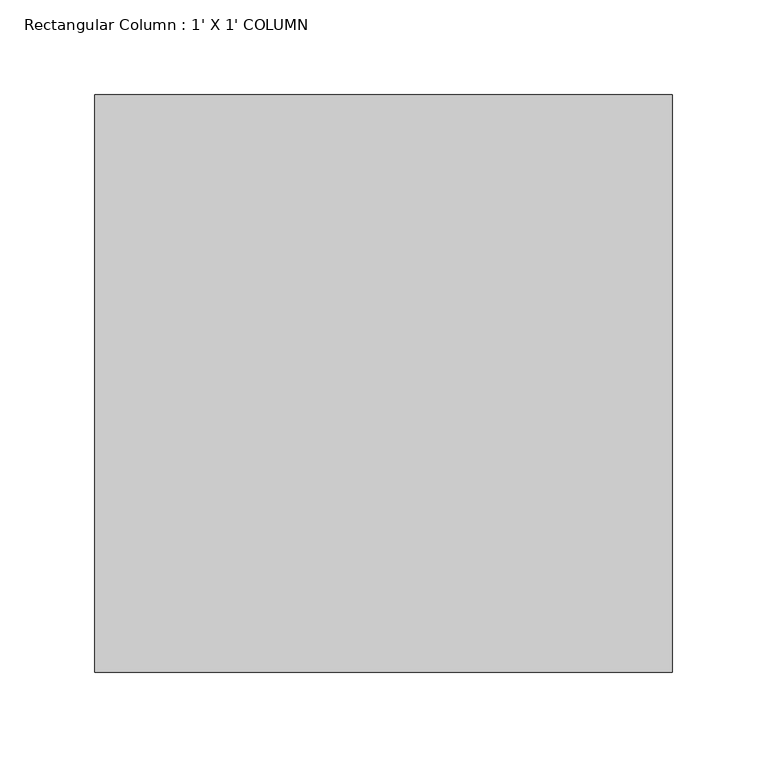
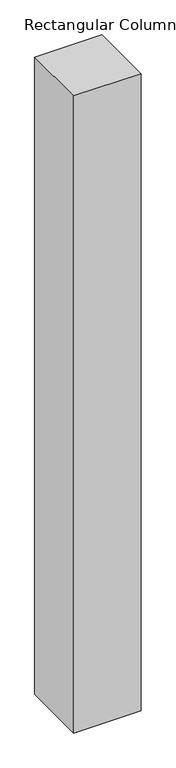
"""IFC4 building model written with IfcOpenShell, lengths in millimetres: column geometry, Rectangular Column : 1' X 1' COLUMN."""

from ifc_helpers import new_model, si_unit, origin, origin_with_axes, place, context, project, spatial, polyline, outline, extrude, source, transform, mapped, element, save


def rectangular_column_1_x_1_column_d780e21f(model_context):
    return source(origin(), model_context, "Body", "SweptSolid", [
        extrude(outline(polyline([(152.4, 152.4), (152.4, -152.4), (-152.4, -152.4), (-152.4, 152.4), (152.4, 152.4)])), origin_with_axes(), (0.0, 0.0, 1.0), 3048.0),
    ])


if __name__ == "__main__":
    model = new_model("IFC4")
    model_context = context("Model", 3, world=origin())
    ifc_project = project(units=[si_unit("LENGTHUNIT", "METRE", prefix="MILLI")], contexts=[model_context])
    site = spatial("IfcSite", under=ifc_project)
    building = spatial("IfcBuilding", under=site)
    placement = place(None, origin())
    rectangular_column_1_x_1_column_shape = rectangular_column_1_x_1_column_d780e21f(model_context)
    element("IfcColumn", 1, ObjectType="Rectangular Column : 1' X 1' COLUMN", at=placement, inside=building, context=model_context, shape_type="MappedRepresentation", body=[
        mapped(rectangular_column_1_x_1_column_shape, transform((0.0, 0.0, 0.0), x_axis=(1.0, 0.0, 0.0), y_axis=(0.0, 1.0, 0.0), z_axis=(0.0, 0.0, 1.0))),
    ])
    save(model, "model.ifc")

# Revit data of these elements
# Type "Rectangular Column : 1' X 1' COLUMN"
#   Assembly Code = "B1010200"
#   Depth = 1' - 0"
#   Offset Base = 0' - 0"
#   Offset Top = 0' - 0"
#   Width = 1' - 0"
#   Material = ROSE COLOUR
# Element 1 (IfcColumn, "Rectangular Column : 1' X 1' COLUMN")
#   Materials on its faces: "ROSE COLOUR"
# Materials
#   "ROSE COLOUR": class "Generic", colour RGB 120 120 120, transparency 0, Cost = 0
